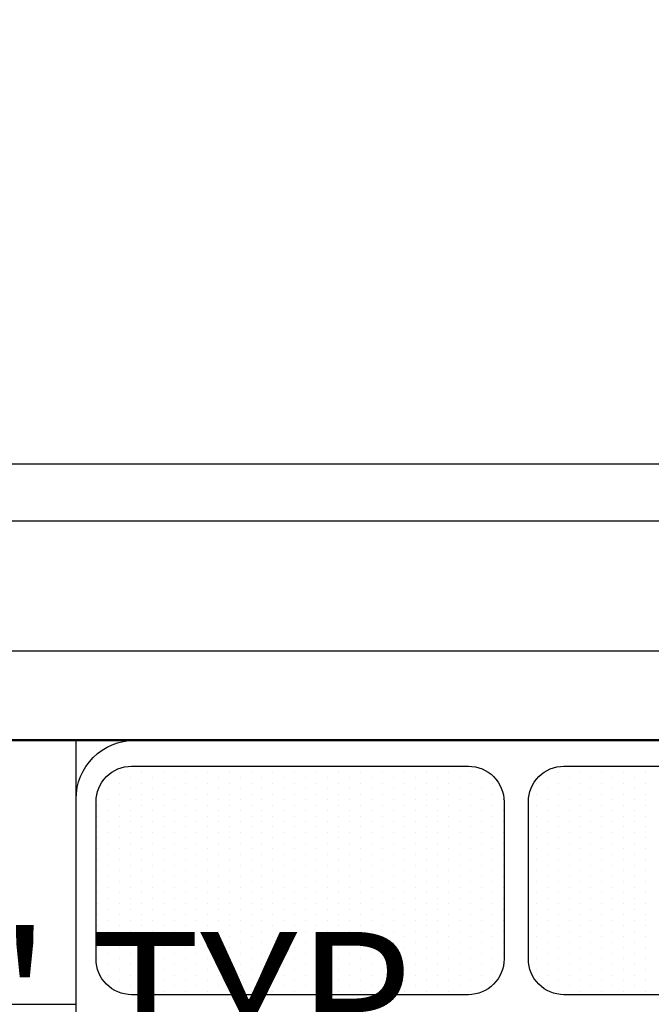
# Model space of a CAD drawing. Units: inches. Extents: x 3064 to 19385, y 846 to 15425.
# Tile 7 of 108: x 3426 to 3469, y 1373 to 1439. Entities that reach past the tile are written whole.
import ezdxf

# ---------------------------------------------------------------- set-up
doc = ezdxf.new("R2010")
doc.units = ezdxf.units.IN
for name, color, linetype, lineweight in [('A-ANNO-DIMS', 2, 'Continuous', 18), ('A-FLOR-FIXT', 9, 'Continuous', 18), ('A-WALL', 7, 'Continuous', 50), ('C-PROP', 6, 'Continuous', 25)]:
    doc.layers.add(name, color=color, linetype=linetype, lineweight=lineweight)
doc.layers.add('BLOCK', color=6, linetype='Continuous')
doc.styles.get("Standard").update_dxf_attribs({"font": 'arial.ttf'})
doc.dimstyles.new('ISO-25', dxfattribs={"dimtxt": 9, "dimasz": 2.5, "dimexe": 1.25, "dimexo": 0.625, "dimtad": 1, "dimdec": 1, "dimlunit": 3, "dimtxsty": 'Standard', "dimcen": 2.5, "dimadec": 0, "dimazin": 0, "dimtfac": 1, "dimtdec": 1, "dimtmove": 0, "dimatfit": 3, "dimfxl": 1, "dimarcsym": 0})

# ---------------------------------------------------------------- blocks, each defined once
blk = doc.blocks.new('*X7')
at = {"color": 0}
for p, q in [((266.25, 456.9375), (266.25, 456.9375)), ((266.4375, 457.03125), (266.4375, 457.03125)), ((266.625, 456.9375), (266.625, 456.9375)), ((266.8125, 457.03125), (266.8125, 457.03125)), ((267, 456.9375), (267, 456.9375)), ((267.1875, 457.03125), (267.1875, 457.03125)), ((267.375, 456.9375), (267.375, 456.9375)), ((267.5625, 457.03125), (267.5625, 457.03125)), ((267.75, 456.9375), (267.75, 456.9375)), ((267.9375, 457.03125), (267.9375, 457.03125)), ((268.125, 456.9375), (268.125, 456.9375)), ((268.3125, 457.03125), (268.3125, 457.03125)), ((268.5, 456.9375), (268.5, 456.9375)), ((268.6875, 457.03125), (268.6875, 457.03125)), ((268.875, 456.9375), (268.875, 456.9375)), ((269.0625, 457.03125), (269.0625, 457.03125)), ((269.25, 456.9375), (269.25, 456.9375)), ((269.4375, 457.03125), (269.4375, 457.03125)), ((269.625, 456.9375), (269.625, 456.9375)), ((269.8125, 457.03125), (269.8125, 457.03125)), ((270, 456.9375), (270, 456.9375)), ((270.1875, 457.03125), (270.1875, 457.03125)), ((270.375, 456.9375), (270.375, 456.9375)), ((270.5625, 457.03125), (270.5625, 457.03125)), ((270.75, 456.9375), (270.75, 456.9375)), ((270.9375, 457.03125), (270.9375, 457.03125)), ((271.125, 456.9375), (271.125, 456.9375)), ((271.3125, 457.03125), (271.3125, 457.03125)), ((271.5, 456.9375), (271.5, 456.9375)), ((271.6875, 457.03125), (271.6875, 457.03125)), ((271.875, 456.9375), (271.875, 456.9375)), ((272.0625, 457.03125), (272.0625, 457.03125)), ((272.25, 456.9375), (272.25, 456.9375)), ((273.75, 456.9375), (273.75, 456.9375)), ((273.9375, 457.03125), (273.9375, 457.03125)), ((274.125, 456.9375), (274.125, 456.9375)), ((274.3125, 457.03125), (274.3125, 457.03125)), ((274.5, 456.9375), (274.5, 456.9375)), ((274.6875, 457.03125), (274.6875, 457.03125)), ((274.875, 456.9375), (274.875, 456.9375)), ((275.0625, 457.03125), (275.0625, 457.03125)), ((275.25, 456.9375), (275.25, 456.9375)), ((266.0625, 456.84375), (266.0625, 456.84375)), ((266.25, 456.75), (266.25, 456.75)), ((266.4375, 456.84375), (266.4375, 456.84375)), ((266.625, 456.75), (266.625, 456.75)), ((266.8125, 456.84375), (266.8125, 456.84375)), ((267, 456.75), (267, 456.75)), ((267.1875, 456.84375), (267.1875, 456.84375)), ((267.375, 456.75), (267.375, 456.75)), ((267.5625, 456.84375), (267.5625, 456.84375)), ((267.75, 456.75), (267.75, 456.75)), ((267.9375, 456.84375), (267.9375, 456.84375)), ((268.125, 456.75), (268.125, 456.75)), ((268.3125, 456.84375), (268.3125, 456.84375)), ((268.5, 456.75), (268.5, 456.75)), ((268.6875, 456.84375), (268.6875, 456.84375)), ((268.875, 456.75), (268.875, 456.75)), ((269.0625, 456.84375), (269.0625, 456.84375)), ((269.25, 456.75), (269.25, 456.75)), ((269.4375, 456.84375), (269.4375, 456.84375)), ((269.625, 456.75), (269.625, 456.75)), ((269.8125, 456.84375), (269.8125, 456.84375)), ((270, 456.75), (270, 456.75)), ((270.1875, 456.84375), (270.1875, 456.84375)), ((270.375, 456.75), (270.375, 456.75)), ((270.5625, 456.84375), (270.5625, 456.84375)), ((270.75, 456.75), (270.75, 456.75)), ((270.9375, 456.84375), (270.9375, 456.84375)), ((271.125, 456.75), (271.125, 456.75)), ((271.3125, 456.84375), (271.3125, 456.84375)), ((271.5, 456.75), (271.5, 456.75)), ((271.6875, 456.84375), (271.6875, 456.84375)), ((271.875, 456.75), (271.875, 456.75)), ((272.0625, 456.84375), (272.0625, 456.84375)), ((272.25, 456.75), (272.25, 456.75)), ((272.4375, 456.84375), (272.4375, 456.84375)), ((272.625, 456.75), (272.625, 456.75)), ((273.375, 456.75), (273.375, 456.75)), ((273.5625, 456.84375), (273.5625, 456.84375)), ((273.75, 456.75), (273.75, 456.75)), ((273.9375, 456.84375), (273.9375, 456.84375)), ((274.125, 456.75), (274.125, 456.75)), ((274.3125, 456.84375), (274.3125, 456.84375)), ((274.5, 456.75), (274.5, 456.75)), ((274.6875, 456.84375), (274.6875, 456.84375)), ((274.875, 456.75), (274.875, 456.75)), ((275.0625, 456.84375), (275.0625, 456.84375)), ((275.25, 456.75), (275.25, 456.75)), ((265.875, 456.5625), (265.875, 456.5625)), ((266.0625, 456.65625), (266.0625, 456.65625)), ((266.25, 456.5625), (266.25, 456.5625)), ((266.4375, 456.65625), (266.4375, 456.65625)), ((266.625, 456.5625), (266.625, 456.5625)), ((266.8125, 456.65625), (266.8125, 456.65625)), ((267, 456.5625), (267, 456.5625)), ((267.1875, 456.65625), (267.1875, 456.65625)), ((267.375, 456.5625), (267.375, 456.5625)), ((267.5625, 456.65625), (267.5625, 456.65625)), ((267.75, 456.5625), (267.75, 456.5625)), ((267.9375, 456.65625), (267.9375, 456.65625)), ((268.125, 456.5625), (268.125, 456.5625)), ((268.3125, 456.65625), (268.3125, 456.65625)), ((268.5, 456.5625), (268.5, 456.5625)), ((268.6875, 456.65625), (268.6875, 456.65625)), ((268.875, 456.5625), (268.875, 456.5625)), ((269.0625, 456.65625), (269.0625, 456.65625)), ((269.25, 456.5625), (269.25, 456.5625)), ((269.4375, 456.65625), (269.4375, 456.65625)), ((269.625, 456.5625), (269.625, 456.5625)), ((269.8125, 456.65625), (269.8125, 456.65625)), ((270, 456.5625), (270, 456.5625)), ((270.1875, 456.65625), (270.1875, 456.65625)), ((270.375, 456.5625), (270.375, 456.5625)), ((270.5625, 456.65625), (270.5625, 456.65625)), ((270.75, 456.5625), (270.75, 456.5625)), ((270.9375, 456.65625), (270.9375, 456.65625)), ((271.125, 456.5625), (271.125, 456.5625)), ((271.3125, 456.65625), (271.3125, 456.65625)), ((271.5, 456.5625), (271.5, 456.5625)), ((271.6875, 456.65625), (271.6875, 456.65625)), ((271.875, 456.5625), (271.875, 456.5625)), ((272.0625, 456.65625), (272.0625, 456.65625)), ((272.25, 456.5625), (272.25, 456.5625)), ((272.4375, 456.65625), (272.4375, 456.65625)), ((272.625, 456.5625), (272.625, 456.5625)), ((273.375, 456.5625), (273.375, 456.5625)), ((273.5625, 456.65625), (273.5625, 456.65625)), ((273.75, 456.5625), (273.75, 456.5625)), ((273.9375, 456.65625), (273.9375, 456.65625)), ((274.125, 456.5625), (274.125, 456.5625)), ((274.3125, 456.65625), (274.3125, 456.65625)), ((274.5, 456.5625), (274.5, 456.5625)), ((274.6875, 456.65625), (274.6875, 456.65625)), ((274.875, 456.5625), (274.875, 456.5625)), ((275.0625, 456.65625), (275.0625, 456.65625)), ((275.25, 456.5625), (275.25, 456.5625)), ((265.875, 456.375), (265.875, 456.375)), ((266.0625, 456.46875), (266.0625, 456.46875)), ((266.25, 456.375), (266.25, 456.375)), ((266.4375, 456.46875), (266.4375, 456.46875)), ((266.625, 456.375), (266.625, 456.375)), ((266.8125, 456.46875), (266.8125, 456.46875)), ((267, 456.375), (267, 456.375)), ((267.1875, 456.46875), (267.1875, 456.46875)), ((267.375, 456.375), (267.375, 456.375)), ((267.5625, 456.46875), (267.5625, 456.46875)), ((267.75, 456.375), (267.75, 456.375)), ((267.9375, 456.46875), (267.9375, 456.46875)), ((268.125, 456.375), (268.125, 456.375)), ((268.3125, 456.46875), (268.3125, 456.46875)), ((268.5, 456.375), (268.5, 456.375)), ((268.6875, 456.46875), (268.6875, 456.46875)), ((268.875, 456.375), (268.875, 456.375)), ((269.0625, 456.46875), (269.0625, 456.46875)), ((269.25, 456.375), (269.25, 456.375)), ((269.4375, 456.46875), (269.4375, 456.46875)), ((269.625, 456.375), (269.625, 456.375)), ((269.8125, 456.46875), (269.8125, 456.46875)), ((270, 456.375), (270, 456.375)), ((270.1875, 456.46875), (270.1875, 456.46875)), ((270.375, 456.375), (270.375, 456.375)), ((270.5625, 456.46875), (270.5625, 456.46875)), ((270.75, 456.375), (270.75, 456.375)), ((270.9375, 456.46875), (270.9375, 456.46875)), ((271.125, 456.375), (271.125, 456.375)), ((271.3125, 456.46875), (271.3125, 456.46875)), ((271.5, 456.375), (271.5, 456.375)), ((271.6875, 456.46875), (271.6875, 456.46875)), ((271.875, 456.375), (271.875, 456.375)), ((272.0625, 456.46875), (272.0625, 456.46875)), ((272.25, 456.375), (272.25, 456.375)), ((272.4375, 456.46875), (272.4375, 456.46875)), ((272.625, 456.375), (272.625, 456.375)), ((272.8125, 456.46875), (272.8125, 456.46875)), ((273.375, 456.375), (273.375, 456.375)), ((273.5625, 456.46875), (273.5625, 456.46875)), ((273.75, 456.375), (273.75, 456.375)), ((273.9375, 456.46875), (273.9375, 456.46875)), ((274.125, 456.375), (274.125, 456.375)), ((274.3125, 456.46875), (274.3125, 456.46875)), ((274.5, 456.375), (274.5, 456.375)), ((274.6875, 456.46875), (274.6875, 456.46875)), ((274.875, 456.375), (274.875, 456.375)), ((275.0625, 456.46875), (275.0625, 456.46875)), ((275.25, 456.375), (275.25, 456.375)), ((266.0625, 456.28125), (266.0625, 456.28125)), ((266.4375, 456.28125), (266.4375, 456.28125)), ((266.8125, 456.28125), (266.8125, 456.28125)), ((267.1875, 456.28125), (267.1875, 456.28125)), ((267.5625, 456.28125), (267.5625, 456.28125)), ((267.9375, 456.28125), (267.9375, 456.28125)), ((268.3125, 456.28125), (268.3125, 456.28125)), ((268.6875, 456.28125), (268.6875, 456.28125)), ((269.0625, 456.28125), (269.0625, 456.28125)), ((269.4375, 456.28125), (269.4375, 456.28125)), ((269.8125, 456.28125), (269.8125, 456.28125)), ((270.1875, 456.28125), (270.1875, 456.28125)), ((270.5625, 456.28125), (270.5625, 456.28125)), ((270.9375, 456.28125), (270.9375, 456.28125)), ((271.3125, 456.28125), (271.3125, 456.28125)), ((271.6875, 456.28125), (271.6875, 456.28125)), ((272.0625, 456.28125), (272.0625, 456.28125)), ((272.4375, 456.28125), (272.4375, 456.28125)), ((272.8125, 456.28125), (272.8125, 456.28125)), ((273.5625, 456.28125), (273.5625, 456.28125)), ((273.9375, 456.28125), (273.9375, 456.28125)), ((274.3125, 456.28125), (274.3125, 456.28125)), ((274.6875, 456.28125), (274.6875, 456.28125)), ((275.0625, 456.28125), (275.0625, 456.28125)), ((265.875, 456.1875), (265.875, 456.1875)), ((266.0625, 456.09375), (266.0625, 456.09375)), ((266.25, 456.1875), (266.25, 456.1875)), ((266.4375, 456.09375), (266.4375, 456.09375)), ((266.625, 456.1875), (266.625, 456.1875)), ((266.8125, 456.09375), (266.8125, 456.09375)), ((267, 456.1875), (267, 456.1875)), ((267.1875, 456.09375), (267.1875, 456.09375)), ((267.375, 456.1875), (267.375, 456.1875)), ((267.5625, 456.09375), (267.5625, 456.09375)), ((267.75, 456.1875), (267.75, 456.1875)), ((267.9375, 456.09375), (267.9375, 456.09375)), ((268.125, 456.1875), (268.125, 456.1875)), ((268.3125, 456.09375), (268.3125, 456.09375)), ((268.5, 456.1875), (268.5, 456.1875)), ((268.6875, 456.09375), (268.6875, 456.09375)), ((268.875, 456.1875), (268.875, 456.1875)), ((269.0625, 456.09375), (269.0625, 456.09375)), ((269.25, 456.1875), (269.25, 456.1875)), ((269.4375, 456.09375), (269.4375, 456.09375)), ((269.625, 456.1875), (269.625, 456.1875)), ((269.8125, 456.09375), (269.8125, 456.09375)), ((270, 456.1875), (270, 456.1875)), ((270.1875, 456.09375), (270.1875, 456.09375)), ((270.375, 456.1875), (270.375, 456.1875)), ((270.5625, 456.09375), (270.5625, 456.09375)), ((270.75, 456.1875), (270.75, 456.1875)), ((270.9375, 456.09375), (270.9375, 456.09375)), ((271.125, 456.1875), (271.125, 456.1875)), ((271.3125, 456.09375), (271.3125, 456.09375)), ((271.5, 456.1875), (271.5, 456.1875)), ((271.6875, 456.09375), (271.6875, 456.09375)), ((271.875, 456.1875), (271.875, 456.1875)), ((272.0625, 456.09375), (272.0625, 456.09375)), ((272.25, 456.1875), (272.25, 456.1875)), ((272.4375, 456.09375), (272.4375, 456.09375)), ((272.625, 456.1875), (272.625, 456.1875)), ((272.8125, 456.09375), (272.8125, 456.09375)), ((273.375, 456.1875), (273.375, 456.1875)), ((273.5625, 456.09375), (273.5625, 456.09375)), ((273.75, 456.1875), (273.75, 456.1875)), ((273.9375, 456.09375), (273.9375, 456.09375)), ((274.125, 456.1875), (274.125, 456.1875)), ((274.3125, 456.09375), (274.3125, 456.09375)), ((274.5, 456.1875), (274.5, 456.1875)), ((274.6875, 456.09375), (274.6875, 456.09375)), ((274.875, 456.1875), (274.875, 456.1875)), ((275.0625, 456.09375), (275.0625, 456.09375)), ((275.25, 456.1875), (275.25, 456.1875)), ((265.875, 456), (265.875, 456)), ((266.0625, 455.90625), (266.0625, 455.90625)), ((266.25, 456), (266.25, 456)), ((266.4375, 455.90625), (266.4375, 455.90625)), ((266.625, 456), (266.625, 456)), ((266.8125, 455.90625), (266.8125, 455.90625)), ((267, 456), (267, 456)), ((267.1875, 455.90625), (267.1875, 455.90625)), ((267.375, 456), (267.375, 456)), ((267.5625, 455.90625), (267.5625, 455.90625)), ((267.75, 456), (267.75, 456)), ((267.9375, 455.90625), (267.9375, 455.90625)), ((268.125, 456), (268.125, 456)), ((268.3125, 455.90625), (268.3125, 455.90625)), ((268.5, 456), (268.5, 456)), ((268.6875, 455.90625), (268.6875, 455.90625)), ((268.875, 456), (268.875, 456)), ((269.0625, 455.90625), (269.0625, 455.90625)), ((269.25, 456), (269.25, 456)), ((269.4375, 455.90625), (269.4375, 455.90625)), ((269.625, 456), (269.625, 456)), ((269.8125, 455.90625), (269.8125, 455.90625)), ((270, 456), (270, 456)), ((270.1875, 455.90625), (270.1875, 455.90625)), ((270.375, 456), (270.375, 456)), ((270.5625, 455.90625), (270.5625, 455.90625)), ((270.75, 456), (270.75, 456)), ((270.9375, 455.90625), (270.9375, 455.90625)), ((271.125, 456), (271.125, 456)), ((271.3125, 455.90625), (271.3125, 455.90625)), ((271.5, 456), (271.5, 456)), ((271.6875, 455.90625), (271.6875, 455.90625)), ((271.875, 456), (271.875, 456)), ((272.0625, 455.90625), (272.0625, 455.90625)), ((272.25, 456), (272.25, 456)), ((272.4375, 455.90625), (272.4375, 455.90625)), ((272.625, 456), (272.625, 456)), ((272.8125, 455.90625), (272.8125, 455.90625)), ((273.375, 456), (273.375, 456)), ((273.5625, 455.90625), (273.5625, 455.90625)), ((273.75, 456), (273.75, 456)), ((273.9375, 455.90625), (273.9375, 455.90625)), ((274.125, 456), (274.125, 456)), ((274.3125, 455.90625), (274.3125, 455.90625)), ((274.5, 456), (274.5, 456)), ((274.6875, 455.90625), (274.6875, 455.90625)), ((274.875, 456), (274.875, 456)), ((275.0625, 455.90625), (275.0625, 455.90625)), ((275.25, 456), (275.25, 456)), ((265.875, 455.8125), (265.875, 455.8125)), ((266.0625, 455.71875), (266.0625, 455.71875)), ((266.25, 455.8125), (266.25, 455.8125)), ((266.4375, 455.71875), (266.4375, 455.71875)), ((266.625, 455.8125), (266.625, 455.8125)), ((266.8125, 455.71875), (266.8125, 455.71875)), ((267, 455.8125), (267, 455.8125)), ((267.1875, 455.71875), (267.1875, 455.71875)), ((267.375, 455.8125), (267.375, 455.8125)), ((267.5625, 455.71875), (267.5625, 455.71875)), ((267.75, 455.8125), (267.75, 455.8125)), ((267.9375, 455.71875), (267.9375, 455.71875)), ((268.125, 455.8125), (268.125, 455.8125)), ((268.3125, 455.71875), (268.3125, 455.71875)), ((268.5, 455.8125), (268.5, 455.8125)), ((268.6875, 455.71875), (268.6875, 455.71875)), ((268.875, 455.8125), (268.875, 455.8125)), ((269.0625, 455.71875), (269.0625, 455.71875)), ((269.25, 455.8125), (269.25, 455.8125)), ((269.4375, 455.71875), (269.4375, 455.71875)), ((269.625, 455.8125), (269.625, 455.8125)), ((269.8125, 455.71875), (269.8125, 455.71875)), ((270, 455.8125), (270, 455.8125)), ((270.1875, 455.71875), (270.1875, 455.71875)), ((270.375, 455.8125), (270.375, 455.8125)), ((270.5625, 455.71875), (270.5625, 455.71875)), ((270.75, 455.8125), (270.75, 455.8125)), ((270.9375, 455.71875), (270.9375, 455.71875)), ((271.125, 455.8125), (271.125, 455.8125)), ((271.3125, 455.71875), (271.3125, 455.71875)), ((271.5, 455.8125), (271.5, 455.8125)), ((271.6875, 455.71875), (271.6875, 455.71875)), ((271.875, 455.8125), (271.875, 455.8125)), ((272.0625, 455.71875), (272.0625, 455.71875)), ((272.25, 455.8125), (272.25, 455.8125)), ((272.4375, 455.71875), (272.4375, 455.71875)), ((272.625, 455.8125), (272.625, 455.8125)), ((272.8125, 455.71875), (272.8125, 455.71875)), ((273.375, 455.8125), (273.375, 455.8125)), ((273.5625, 455.71875), (273.5625, 455.71875)), ((273.75, 455.8125), (273.75, 455.8125)), ((273.9375, 455.71875), (273.9375, 455.71875)), ((274.125, 455.8125), (274.125, 455.8125)), ((274.3125, 455.71875), (274.3125, 455.71875)), ((274.5, 455.8125), (274.5, 455.8125)), ((274.6875, 455.71875), (274.6875, 455.71875)), ((274.875, 455.8125), (274.875, 455.8125)), ((275.0625, 455.71875), (275.0625, 455.71875)), ((275.25, 455.8125), (275.25, 455.8125)), ((265.875, 455.625), (265.875, 455.625)), ((266.0625, 455.53125), (266.0625, 455.53125)), ((266.25, 455.625), (266.25, 455.625)), ((266.4375, 455.53125), (266.4375, 455.53125)), ((266.625, 455.625), (266.625, 455.625)), ((266.8125, 455.53125), (266.8125, 455.53125)), ((267, 455.625), (267, 455.625)), ((267.1875, 455.53125), (267.1875, 455.53125)), ((267.375, 455.625), (267.375, 455.625)), ((267.5625, 455.53125), (267.5625, 455.53125)), ((267.75, 455.625), (267.75, 455.625)), ((267.9375, 455.53125), (267.9375, 455.53125)), ((268.125, 455.625), (268.125, 455.625)), ((268.3125, 455.53125), (268.3125, 455.53125)), ((268.5, 455.625), (268.5, 455.625)), ((268.6875, 455.53125), (268.6875, 455.53125)), ((268.875, 455.625), (268.875, 455.625)), ((269.0625, 455.53125), (269.0625, 455.53125)), ((269.25, 455.625), (269.25, 455.625)), ((269.4375, 455.53125), (269.4375, 455.53125)), ((269.625, 455.625), (269.625, 455.625)), ((269.8125, 455.53125), (269.8125, 455.53125)), ((270, 455.625), (270, 455.625)), ((270.1875, 455.53125), (270.1875, 455.53125)), ((270.375, 455.625), (270.375, 455.625)), ((270.5625, 455.53125), (270.5625, 455.53125)), ((270.75, 455.625), (270.75, 455.625)), ((270.9375, 455.53125), (270.9375, 455.53125)), ((271.125, 455.625), (271.125, 455.625)), ((271.3125, 455.53125), (271.3125, 455.53125)), ((271.5, 455.625), (271.5, 455.625)), ((271.6875, 455.53125), (271.6875, 455.53125)), ((271.875, 455.625), (271.875, 455.625)), ((272.0625, 455.53125), (272.0625, 455.53125)), ((272.25, 455.625), (272.25, 455.625)), ((272.4375, 455.53125), (272.4375, 455.53125)), ((272.625, 455.625), (272.625, 455.625)), ((272.8125, 455.53125), (272.8125, 455.53125)), ((273.375, 455.625), (273.375, 455.625)), ((273.5625, 455.53125), (273.5625, 455.53125)), ((273.75, 455.625), (273.75, 455.625)), ((273.9375, 455.53125), (273.9375, 455.53125)), ((274.125, 455.625), (274.125, 455.625)), ((274.3125, 455.53125), (274.3125, 455.53125)), ((274.5, 455.625), (274.5, 455.625)), ((274.6875, 455.53125), (274.6875, 455.53125)), ((274.875, 455.625), (274.875, 455.625)), ((275.0625, 455.53125), (275.0625, 455.53125)), ((275.25, 455.625), (275.25, 455.625)), ((265.875, 455.4375), (265.875, 455.4375)), ((266.25, 455.4375), (266.25, 455.4375)), ((266.625, 455.4375), (266.625, 455.4375)), ((267, 455.4375), (267, 455.4375)), ((267.375, 455.4375), (267.375, 455.4375)), ((267.75, 455.4375), (267.75, 455.4375)), ((268.125, 455.4375), (268.125, 455.4375)), ((268.5, 455.4375), (268.5, 455.4375)), ((268.875, 455.4375), (268.875, 455.4375)), ((269.25, 455.4375), (269.25, 455.4375)), ((269.625, 455.4375), (269.625, 455.4375)), ((270, 455.4375), (270, 455.4375)), ((270.375, 455.4375), (270.375, 455.4375)), ((270.75, 455.4375), (270.75, 455.4375)), ((271.125, 455.4375), (271.125, 455.4375)), ((271.5, 455.4375), (271.5, 455.4375)), ((271.875, 455.4375), (271.875, 455.4375)), ((272.25, 455.4375), (272.25, 455.4375)), ((272.625, 455.4375), (272.625, 455.4375)), ((273.375, 455.4375), (273.375, 455.4375)), ((273.75, 455.4375), (273.75, 455.4375)), ((274.125, 455.4375), (274.125, 455.4375)), ((274.5, 455.4375), (274.5, 455.4375)), ((274.875, 455.4375), (274.875, 455.4375)), ((275.25, 455.4375), (275.25, 455.4375)), ((265.875, 455.25), (265.875, 455.25)), ((266.0625, 455.34375), (266.0625, 455.34375)), ((266.25, 455.25), (266.25, 455.25)), ((266.4375, 455.34375), (266.4375, 455.34375)), ((266.625, 455.25), (266.625, 455.25)), ((266.8125, 455.34375), (266.8125, 455.34375)), ((267, 455.25), (267, 455.25)), ((267.1875, 455.34375), (267.1875, 455.34375)), ((267.375, 455.25), (267.375, 455.25)), ((267.5625, 455.34375), (267.5625, 455.34375)), ((267.75, 455.25), (267.75, 455.25)), ((267.9375, 455.34375), (267.9375, 455.34375)), ((268.125, 455.25), (268.125, 455.25)), ((268.3125, 455.34375), (268.3125, 455.34375)), ((268.5, 455.25), (268.5, 455.25)), ((268.6875, 455.34375), (268.6875, 455.34375)), ((268.875, 455.25), (268.875, 455.25)), ((269.0625, 455.34375), (269.0625, 455.34375)), ((269.25, 455.25), (269.25, 455.25)), ((269.4375, 455.34375), (269.4375, 455.34375)), ((269.625, 455.25), (269.625, 455.25)), ((269.8125, 455.34375), (269.8125, 455.34375)), ((270, 455.25), (270, 455.25)), ((270.1875, 455.34375), (270.1875, 455.34375)), ((270.375, 455.25), (270.375, 455.25)), ((270.5625, 455.34375), (270.5625, 455.34375)), ((270.75, 455.25), (270.75, 455.25)), ((270.9375, 455.34375), (270.9375, 455.34375)), ((271.125, 455.25), (271.125, 455.25)), ((271.3125, 455.34375), (271.3125, 455.34375)), ((271.5, 455.25), (271.5, 455.25)), ((271.6875, 455.34375), (271.6875, 455.34375)), ((271.875, 455.25), (271.875, 455.25)), ((272.0625, 455.34375), (272.0625, 455.34375)), ((272.25, 455.25), (272.25, 455.25)), ((272.4375, 455.34375), (272.4375, 455.34375)), ((272.625, 455.25), (272.625, 455.25)), ((272.8125, 455.34375), (272.8125, 455.34375)), ((273.375, 455.25), (273.375, 455.25)), ((273.5625, 455.34375), (273.5625, 455.34375)), ((273.75, 455.25), (273.75, 455.25)), ((273.9375, 455.34375), (273.9375, 455.34375)), ((274.125, 455.25), (274.125, 455.25)), ((274.3125, 455.34375), (274.3125, 455.34375)), ((274.5, 455.25), (274.5, 455.25)), ((274.6875, 455.34375), (274.6875, 455.34375)), ((274.875, 455.25), (274.875, 455.25)), ((275.0625, 455.34375), (275.0625, 455.34375)), ((275.25, 455.25), (275.25, 455.25)), ((265.875, 455.0625), (265.875, 455.0625)), ((266.0625, 455.15625), (266.0625, 455.15625)), ((266.25, 455.0625), (266.25, 455.0625)), ((266.4375, 455.15625), (266.4375, 455.15625)), ((266.625, 455.0625), (266.625, 455.0625)), ((266.8125, 455.15625), (266.8125, 455.15625)), ((267, 455.0625), (267, 455.0625)), ((267.1875, 455.15625), (267.1875, 455.15625)), ((267.375, 455.0625), (267.375, 455.0625)), ((267.5625, 455.15625), (267.5625, 455.15625)), ((267.75, 455.0625), (267.75, 455.0625)), ((267.9375, 455.15625), (267.9375, 455.15625)), ((268.125, 455.0625), (268.125, 455.0625)), ((268.3125, 455.15625), (268.3125, 455.15625)), ((268.5, 455.0625), (268.5, 455.0625)), ((268.6875, 455.15625), (268.6875, 455.15625)), ((268.875, 455.0625), (268.875, 455.0625)), ((269.0625, 455.15625), (269.0625, 455.15625)), ((269.25, 455.0625), (269.25, 455.0625)), ((269.4375, 455.15625), (269.4375, 455.15625)), ((269.625, 455.0625), (269.625, 455.0625)), ((269.8125, 455.15625), (269.8125, 455.15625)), ((270, 455.0625), (270, 455.0625)), ((270.1875, 455.15625), (270.1875, 455.15625)), ((270.375, 455.0625), (270.375, 455.0625)), ((270.5625, 455.15625), (270.5625, 455.15625)), ((270.75, 455.0625), (270.75, 455.0625)), ((270.9375, 455.15625), (270.9375, 455.15625)), ((271.125, 455.0625), (271.125, 455.0625)), ((271.3125, 455.15625), (271.3125, 455.15625)), ((271.5, 455.0625), (271.5, 455.0625)), ((271.6875, 455.15625), (271.6875, 455.15625)), ((271.875, 455.0625), (271.875, 455.0625)), ((272.0625, 455.15625), (272.0625, 455.15625)), ((272.25, 455.0625), (272.25, 455.0625)), ((272.4375, 455.15625), (272.4375, 455.15625)), ((272.625, 455.0625), (272.625, 455.0625)), ((272.8125, 455.15625), (272.8125, 455.15625)), ((273.375, 455.0625), (273.375, 455.0625)), ((273.5625, 455.15625), (273.5625, 455.15625)), ((273.75, 455.0625), (273.75, 455.0625)), ((273.9375, 455.15625), (273.9375, 455.15625)), ((274.125, 455.0625), (274.125, 455.0625)), ((274.3125, 455.15625), (274.3125, 455.15625)), ((274.5, 455.0625), (274.5, 455.0625)), ((274.6875, 455.15625), (274.6875, 455.15625)), ((274.875, 455.0625), (274.875, 455.0625)), ((275.0625, 455.15625), (275.0625, 455.15625)), ((275.25, 455.0625), (275.25, 455.0625)), ((265.875, 454.875), (265.875, 454.875)), ((266.0625, 454.96875), (266.0625, 454.96875)), ((266.25, 454.875), (266.25, 454.875)), ((266.4375, 454.96875), (266.4375, 454.96875)), ((266.625, 454.875), (266.625, 454.875)), ((266.8125, 454.96875), (266.8125, 454.96875)), ((267, 454.875), (267, 454.875)), ((267.1875, 454.96875), (267.1875, 454.96875)), ((267.375, 454.875), (267.375, 454.875)), ((267.5625, 454.96875), (267.5625, 454.96875)), ((267.75, 454.875), (267.75, 454.875)), ((267.9375, 454.96875), (267.9375, 454.96875)), ((268.125, 454.875), (268.125, 454.875)), ((268.3125, 454.96875), (268.3125, 454.96875)), ((268.5, 454.875), (268.5, 454.875)), ((268.6875, 454.96875), (268.6875, 454.96875)), ((268.875, 454.875), (268.875, 454.875)), ((269.0625, 454.96875), (269.0625, 454.96875)), ((269.25, 454.875), (269.25, 454.875)), ((269.4375, 454.96875), (269.4375, 454.96875)), ((269.625, 454.875), (269.625, 454.875)), ((269.8125, 454.96875), (269.8125, 454.96875)), ((270, 454.875), (270, 454.875)), ((270.1875, 454.96875), (270.1875, 454.96875)), ((270.375, 454.875), (270.375, 454.875)), ((270.5625, 454.96875), (270.5625, 454.96875)), ((270.75, 454.875), (270.75, 454.875)), ((270.9375, 454.96875), (270.9375, 454.96875)), ((271.125, 454.875), (271.125, 454.875)), ((271.3125, 454.96875), (271.3125, 454.96875)), ((271.5, 454.875), (271.5, 454.875)), ((271.6875, 454.96875), (271.6875, 454.96875)), ((271.875, 454.875), (271.875, 454.875)), ((272.0625, 454.96875), (272.0625, 454.96875)), ((272.25, 454.875), (272.25, 454.875)), ((272.4375, 454.96875), (272.4375, 454.96875)), ((272.625, 454.875), (272.625, 454.875)), ((272.8125, 454.96875), (272.8125, 454.96875)), ((273.375, 454.875), (273.375, 454.875)), ((273.5625, 454.96875), (273.5625, 454.96875)), ((273.75, 454.875), (273.75, 454.875)), ((273.9375, 454.96875), (273.9375, 454.96875)), ((274.125, 454.875), (274.125, 454.875)), ((274.3125, 454.96875), (274.3125, 454.96875)), ((274.5, 454.875), (274.5, 454.875)), ((274.6875, 454.96875), (274.6875, 454.96875)), ((274.875, 454.875), (274.875, 454.875)), ((275.0625, 454.96875), (275.0625, 454.96875)), ((275.25, 454.875), (275.25, 454.875)), ((265.875, 454.6875), (265.875, 454.6875)), ((266.0625, 454.78125), (266.0625, 454.78125)), ((266.25, 454.6875), (266.25, 454.6875)), ((266.4375, 454.78125), (266.4375, 454.78125)), ((266.625, 454.6875), (266.625, 454.6875)), ((266.8125, 454.78125), (266.8125, 454.78125)), ((267, 454.6875), (267, 454.6875)), ((267.1875, 454.78125), (267.1875, 454.78125)), ((267.375, 454.6875), (267.375, 454.6875)), ((267.5625, 454.78125), (267.5625, 454.78125)), ((267.75, 454.6875), (267.75, 454.6875)), ((267.9375, 454.78125), (267.9375, 454.78125)), ((268.125, 454.6875), (268.125, 454.6875)), ((268.3125, 454.78125), (268.3125, 454.78125)), ((268.5, 454.6875), (268.5, 454.6875)), ((268.6875, 454.78125), (268.6875, 454.78125)), ((268.875, 454.6875), (268.875, 454.6875)), ((269.0625, 454.78125), (269.0625, 454.78125)), ((269.25, 454.6875), (269.25, 454.6875)), ((269.4375, 454.78125), (269.4375, 454.78125)), ((269.625, 454.6875), (269.625, 454.6875)), ((269.8125, 454.78125), (269.8125, 454.78125)), ((270, 454.6875), (270, 454.6875)), ((270.1875, 454.78125), (270.1875, 454.78125)), ((270.375, 454.6875), (270.375, 454.6875)), ((270.5625, 454.78125), (270.5625, 454.78125)), ((270.75, 454.6875), (270.75, 454.6875)), ((270.9375, 454.78125), (270.9375, 454.78125)), ((271.125, 454.6875), (271.125, 454.6875)), ((271.3125, 454.78125), (271.3125, 454.78125)), ((271.5, 454.6875), (271.5, 454.6875)), ((271.6875, 454.78125), (271.6875, 454.78125)), ((271.875, 454.6875), (271.875, 454.6875)), ((272.0625, 454.78125), (272.0625, 454.78125)), ((272.25, 454.6875), (272.25, 454.6875)), ((272.4375, 454.78125), (272.4375, 454.78125)), ((272.625, 454.6875), (272.625, 454.6875)), ((272.8125, 454.78125), (272.8125, 454.78125)), ((273.375, 454.6875), (273.375, 454.6875)), ((273.5625, 454.78125), (273.5625, 454.78125)), ((273.75, 454.6875), (273.75, 454.6875)), ((273.9375, 454.78125), (273.9375, 454.78125)), ((274.125, 454.6875), (274.125, 454.6875)), ((274.3125, 454.78125), (274.3125, 454.78125)), ((274.5, 454.6875), (274.5, 454.6875)), ((274.6875, 454.78125), (274.6875, 454.78125)), ((274.875, 454.6875), (274.875, 454.6875)), ((275.0625, 454.78125), (275.0625, 454.78125)), ((275.25, 454.6875), (275.25, 454.6875)), ((266.0625, 454.59375), (266.0625, 454.59375)), ((266.4375, 454.59375), (266.4375, 454.59375)), ((266.8125, 454.59375), (266.8125, 454.59375)), ((267.1875, 454.59375), (267.1875, 454.59375)), ((267.5625, 454.59375), (267.5625, 454.59375)), ((267.9375, 454.59375), (267.9375, 454.59375)), ((268.3125, 454.59375), (268.3125, 454.59375)), ((268.6875, 454.59375), (268.6875, 454.59375)), ((269.0625, 454.59375), (269.0625, 454.59375)), ((269.4375, 454.59375), (269.4375, 454.59375)), ((269.8125, 454.59375), (269.8125, 454.59375)), ((270.1875, 454.59375), (270.1875, 454.59375)), ((270.5625, 454.59375), (270.5625, 454.59375)), ((270.9375, 454.59375), (270.9375, 454.59375)), ((271.3125, 454.59375), (271.3125, 454.59375)), ((271.6875, 454.59375), (271.6875, 454.59375)), ((272.0625, 454.59375), (272.0625, 454.59375)), ((272.4375, 454.59375), (272.4375, 454.59375)), ((272.8125, 454.59375), (272.8125, 454.59375)), ((273.5625, 454.59375), (273.5625, 454.59375)), ((273.9375, 454.59375), (273.9375, 454.59375)), ((274.3125, 454.59375), (274.3125, 454.59375)), ((274.6875, 454.59375), (274.6875, 454.59375)), ((275.0625, 454.59375), (275.0625, 454.59375)), ((265.875, 454.5), (265.875, 454.5)), ((266.0625, 454.40625), (266.0625, 454.40625)), ((266.25, 454.5), (266.25, 454.5)), ((266.4375, 454.40625), (266.4375, 454.40625)), ((266.625, 454.5), (266.625, 454.5)), ((266.8125, 454.40625), (266.8125, 454.40625)), ((267, 454.5), (267, 454.5)), ((267.1875, 454.40625), (267.1875, 454.40625)), ((267.375, 454.5), (267.375, 454.5)), ((267.5625, 454.40625), (267.5625, 454.40625)), ((267.75, 454.5), (267.75, 454.5)), ((267.9375, 454.40625), (267.9375, 454.40625)), ((268.125, 454.5), (268.125, 454.5)), ((268.3125, 454.40625), (268.3125, 454.40625)), ((268.5, 454.5), (268.5, 454.5)), ((268.6875, 454.40625), (268.6875, 454.40625)), ((268.875, 454.5), (268.875, 454.5)), ((269.0625, 454.40625), (269.0625, 454.40625)), ((269.25, 454.5), (269.25, 454.5)), ((269.4375, 454.40625), (269.4375, 454.40625)), ((269.625, 454.5), (269.625, 454.5)), ((269.8125, 454.40625), (269.8125, 454.40625)), ((270, 454.5), (270, 454.5)), ((270.1875, 454.40625), (270.1875, 454.40625)), ((270.375, 454.5), (270.375, 454.5)), ((270.5625, 454.40625), (270.5625, 454.40625)), ((270.75, 454.5), (270.75, 454.5)), ((270.9375, 454.40625), (270.9375, 454.40625)), ((271.125, 454.5), (271.125, 454.5)), ((271.3125, 454.40625), (271.3125, 454.40625)), ((271.5, 454.5), (271.5, 454.5)), ((271.6875, 454.40625), (271.6875, 454.40625)), ((271.875, 454.5), (271.875, 454.5)), ((272.0625, 454.40625), (272.0625, 454.40625)), ((272.25, 454.5), (272.25, 454.5)), ((272.4375, 454.40625), (272.4375, 454.40625)), ((272.625, 454.5), (272.625, 454.5)), ((272.8125, 454.40625), (272.8125, 454.40625)), ((273.375, 454.5), (273.375, 454.5)), ((273.5625, 454.40625), (273.5625, 454.40625)), ((273.75, 454.5), (273.75, 454.5)), ((273.9375, 454.40625), (273.9375, 454.40625)), ((274.125, 454.5), (274.125, 454.5)), ((274.3125, 454.40625), (274.3125, 454.40625)), ((274.5, 454.5), (274.5, 454.5)), ((274.6875, 454.40625), (274.6875, 454.40625)), ((274.875, 454.5), (274.875, 454.5)), ((275.0625, 454.40625), (275.0625, 454.40625)), ((275.25, 454.5), (275.25, 454.5)), ((265.875, 454.3125), (265.875, 454.3125)), ((266.0625, 454.21875), (266.0625, 454.21875)), ((266.25, 454.3125), (266.25, 454.3125)), ((266.4375, 454.21875), (266.4375, 454.21875)), ((266.625, 454.3125), (266.625, 454.3125)), ((266.8125, 454.21875), (266.8125, 454.21875)), ((267, 454.3125), (267, 454.3125)), ((267.1875, 454.21875), (267.1875, 454.21875)), ((267.375, 454.3125), (267.375, 454.3125)), ((267.5625, 454.21875), (267.5625, 454.21875)), ((267.75, 454.3125), (267.75, 454.3125)), ((267.9375, 454.21875), (267.9375, 454.21875)), ((268.125, 454.3125), (268.125, 454.3125)), ((268.3125, 454.21875), (268.3125, 454.21875)), ((268.5, 454.3125), (268.5, 454.3125)), ((268.6875, 454.21875), (268.6875, 454.21875)), ((268.875, 454.3125), (268.875, 454.3125)), ((269.0625, 454.21875), (269.0625, 454.21875)), ((269.25, 454.3125), (269.25, 454.3125)), ((269.4375, 454.21875), (269.4375, 454.21875)), ((269.625, 454.3125), (269.625, 454.3125)), ((269.8125, 454.21875), (269.8125, 454.21875)), ((270, 454.3125), (270, 454.3125)), ((270.1875, 454.21875), (270.1875, 454.21875)), ((270.375, 454.3125), (270.375, 454.3125)), ((270.5625, 454.21875), (270.5625, 454.21875)), ((270.75, 454.3125), (270.75, 454.3125)), ((270.9375, 454.21875), (270.9375, 454.21875)), ((271.125, 454.3125), (271.125, 454.3125)), ((271.3125, 454.21875), (271.3125, 454.21875)), ((271.5, 454.3125), (271.5, 454.3125)), ((271.6875, 454.21875), (271.6875, 454.21875)), ((271.875, 454.3125), (271.875, 454.3125)), ((272.0625, 454.21875), (272.0625, 454.21875)), ((272.25, 454.3125), (272.25, 454.3125)), ((272.4375, 454.21875), (272.4375, 454.21875)), ((272.625, 454.3125), (272.625, 454.3125)), ((272.8125, 454.21875), (272.8125, 454.21875)), ((273.375, 454.3125), (273.375, 454.3125)), ((273.5625, 454.21875), (273.5625, 454.21875)), ((273.75, 454.3125), (273.75, 454.3125)), ((273.9375, 454.21875), (273.9375, 454.21875)), ((274.125, 454.3125), (274.125, 454.3125)), ((274.3125, 454.21875), (274.3125, 454.21875)), ((274.5, 454.3125), (274.5, 454.3125)), ((274.6875, 454.21875), (274.6875, 454.21875)), ((274.875, 454.3125), (274.875, 454.3125)), ((275.0625, 454.21875), (275.0625, 454.21875)), ((275.25, 454.3125), (275.25, 454.3125)), ((265.875, 454.125), (265.875, 454.125)), ((266.0625, 454.03125), (266.0625, 454.03125)), ((266.25, 454.125), (266.25, 454.125)), ((266.4375, 454.03125), (266.4375, 454.03125)), ((266.625, 454.125), (266.625, 454.125)), ((266.8125, 454.03125), (266.8125, 454.03125)), ((267, 454.125), (267, 454.125)), ((267.1875, 454.03125), (267.1875, 454.03125)), ((267.375, 454.125), (267.375, 454.125)), ((267.5625, 454.03125), (267.5625, 454.03125)), ((267.75, 454.125), (267.75, 454.125)), ((267.9375, 454.03125), (267.9375, 454.03125)), ((268.125, 454.125), (268.125, 454.125)), ((268.3125, 454.03125), (268.3125, 454.03125)), ((268.5, 454.125), (268.5, 454.125)), ((268.6875, 454.03125), (268.6875, 454.03125)), ((268.875, 454.125), (268.875, 454.125)), ((269.0625, 454.03125), (269.0625, 454.03125)), ((269.25, 454.125), (269.25, 454.125)), ((269.4375, 454.03125), (269.4375, 454.03125)), ((269.625, 454.125), (269.625, 454.125)), ((269.8125, 454.03125), (269.8125, 454.03125)), ((270, 454.125), (270, 454.125)), ((270.1875, 454.03125), (270.1875, 454.03125)), ((270.375, 454.125), (270.375, 454.125)), ((270.5625, 454.03125), (270.5625, 454.03125)), ((270.75, 454.125), (270.75, 454.125)), ((270.9375, 454.03125), (270.9375, 454.03125)), ((271.125, 454.125), (271.125, 454.125)), ((271.3125, 454.03125), (271.3125, 454.03125)), ((271.5, 454.125), (271.5, 454.125)), ((271.6875, 454.03125), (271.6875, 454.03125)), ((271.875, 454.125), (271.875, 454.125)), ((272.0625, 454.03125), (272.0625, 454.03125)), ((272.25, 454.125), (272.25, 454.125)), ((272.4375, 454.03125), (272.4375, 454.03125)), ((272.625, 454.125), (272.625, 454.125)), ((272.8125, 454.03125), (272.8125, 454.03125)), ((273.375, 454.125), (273.375, 454.125)), ((273.5625, 454.03125), (273.5625, 454.03125)), ((273.75, 454.125), (273.75, 454.125)), ((273.9375, 454.03125), (273.9375, 454.03125)), ((274.125, 454.125), (274.125, 454.125)), ((274.3125, 454.03125), (274.3125, 454.03125)), ((274.5, 454.125), (274.5, 454.125)), ((274.6875, 454.03125), (274.6875, 454.03125)), ((274.875, 454.125), (274.875, 454.125)), ((275.0625, 454.03125), (275.0625, 454.03125)), ((275.25, 454.125), (275.25, 454.125)), ((265.875, 453.9375), (265.875, 453.9375)), ((266.25, 453.9375), (266.25, 453.9375)), ((266.625, 453.9375), (266.625, 453.9375)), ((267, 453.9375), (267, 453.9375)), ((267.375, 453.9375), (267.375, 453.9375)), ((267.75, 453.9375), (267.75, 453.9375)), ((268.125, 453.9375), (268.125, 453.9375)), ((268.5, 453.9375), (268.5, 453.9375)), ((268.875, 453.9375), (268.875, 453.9375)), ((269.25, 453.9375), (269.25, 453.9375)), ((269.625, 453.9375), (269.625, 453.9375)), ((270, 453.9375), (270, 453.9375)), ((270.375, 453.9375), (270.375, 453.9375)), ((270.75, 453.9375), (270.75, 453.9375)), ((271.125, 453.9375), (271.125, 453.9375)), ((271.5, 453.9375), (271.5, 453.9375)), ((271.875, 453.9375), (271.875, 453.9375)), ((272.25, 453.9375), (272.25, 453.9375)), ((272.625, 453.9375), (272.625, 453.9375)), ((273.375, 453.9375), (273.375, 453.9375)), ((273.75, 453.9375), (273.75, 453.9375)), ((274.125, 453.9375), (274.125, 453.9375)), ((274.5, 453.9375), (274.5, 453.9375)), ((274.875, 453.9375), (274.875, 453.9375)), ((275.25, 453.9375), (275.25, 453.9375)), ((265.875, 453.75), (265.875, 453.75)), ((266.0625, 453.84375), (266.0625, 453.84375)), ((266.25, 453.75), (266.25, 453.75)), ((266.4375, 453.84375), (266.4375, 453.84375)), ((266.625, 453.75), (266.625, 453.75)), ((266.8125, 453.84375), (266.8125, 453.84375)), ((267, 453.75), (267, 453.75)), ((267.1875, 453.84375), (267.1875, 453.84375)), ((267.375, 453.75), (267.375, 453.75)), ((267.5625, 453.84375), (267.5625, 453.84375)), ((267.75, 453.75), (267.75, 453.75)), ((267.9375, 453.84375), (267.9375, 453.84375)), ((268.125, 453.75), (268.125, 453.75)), ((268.3125, 453.84375), (268.3125, 453.84375)), ((268.5, 453.75), (268.5, 453.75)), ((268.6875, 453.84375), (268.6875, 453.84375)), ((268.875, 453.75), (268.875, 453.75)), ((269.0625, 453.84375), (269.0625, 453.84375)), ((269.25, 453.75), (269.25, 453.75)), ((269.4375, 453.84375), (269.4375, 453.84375)), ((269.625, 453.75), (269.625, 453.75)), ((269.8125, 453.84375), (269.8125, 453.84375)), ((270, 453.75), (270, 453.75)), ((270.1875, 453.84375), (270.1875, 453.84375)), ((270.375, 453.75), (270.375, 453.75)), ((270.5625, 453.84375), (270.5625, 453.84375)), ((270.75, 453.75), (270.75, 453.75)), ((270.9375, 453.84375), (270.9375, 453.84375)), ((271.125, 453.75), (271.125, 453.75)), ((271.3125, 453.84375), (271.3125, 453.84375)), ((271.5, 453.75), (271.5, 453.75)), ((271.6875, 453.84375), (271.6875, 453.84375)), ((271.875, 453.75), (271.875, 453.75)), ((272.0625, 453.84375), (272.0625, 453.84375)), ((272.25, 453.75), (272.25, 453.75)), ((272.4375, 453.84375), (272.4375, 453.84375)), ((272.625, 453.75), (272.625, 453.75)), ((272.8125, 453.84375), (272.8125, 453.84375)), ((273.375, 453.75), (273.375, 453.75)), ((273.5625, 453.84375), (273.5625, 453.84375)), ((273.75, 453.75), (273.75, 453.75)), ((273.9375, 453.84375), (273.9375, 453.84375)), ((274.125, 453.75), (274.125, 453.75)), ((274.3125, 453.84375), (274.3125, 453.84375)), ((274.5, 453.75), (274.5, 453.75)), ((274.6875, 453.84375), (274.6875, 453.84375)), ((274.875, 453.75), (274.875, 453.75)), ((275.0625, 453.84375), (275.0625, 453.84375)), ((275.25, 453.75), (275.25, 453.75)), ((266.0625, 453.65625), (266.0625, 453.65625)), ((266.25, 453.5625), (266.25, 453.5625)), ((266.4375, 453.65625), (266.4375, 453.65625)), ((266.625, 453.5625), (266.625, 453.5625)), ((266.8125, 453.65625), (266.8125, 453.65625)), ((267, 453.5625), (267, 453.5625)), ((267.1875, 453.65625), (267.1875, 453.65625)), ((267.375, 453.5625), (267.375, 453.5625)), ((267.5625, 453.65625), (267.5625, 453.65625)), ((267.75, 453.5625), (267.75, 453.5625)), ((267.9375, 453.65625), (267.9375, 453.65625)), ((268.125, 453.5625), (268.125, 453.5625)), ((268.3125, 453.65625), (268.3125, 453.65625)), ((268.5, 453.5625), (268.5, 453.5625)), ((268.6875, 453.65625), (268.6875, 453.65625)), ((268.875, 453.5625), (268.875, 453.5625)), ((269.0625, 453.65625), (269.0625, 453.65625)), ((269.25, 453.5625), (269.25, 453.5625)), ((269.4375, 453.65625), (269.4375, 453.65625)), ((269.625, 453.5625), (269.625, 453.5625)), ((269.8125, 453.65625), (269.8125, 453.65625)), ((270, 453.5625), (270, 453.5625)), ((270.1875, 453.65625), (270.1875, 453.65625)), ((270.375, 453.5625), (270.375, 453.5625)), ((270.5625, 453.65625), (270.5625, 453.65625)), ((270.75, 453.5625), (270.75, 453.5625)), ((270.9375, 453.65625), (270.9375, 453.65625)), ((271.125, 453.5625), (271.125, 453.5625)), ((271.3125, 453.65625), (271.3125, 453.65625)), ((271.5, 453.5625), (271.5, 453.5625)), ((271.6875, 453.65625), (271.6875, 453.65625)), ((271.875, 453.5625), (271.875, 453.5625)), ((272.0625, 453.65625), (272.0625, 453.65625)), ((272.25, 453.5625), (272.25, 453.5625)), ((272.4375, 453.65625), (272.4375, 453.65625)), ((272.625, 453.5625), (272.625, 453.5625)), ((272.8125, 453.65625), (272.8125, 453.65625)), ((273.375, 453.5625), (273.375, 453.5625)), ((273.5625, 453.65625), (273.5625, 453.65625)), ((273.75, 453.5625), (273.75, 453.5625)), ((273.9375, 453.65625), (273.9375, 453.65625)), ((274.125, 453.5625), (274.125, 453.5625)), ((274.3125, 453.65625), (274.3125, 453.65625)), ((274.5, 453.5625), (274.5, 453.5625)), ((274.6875, 453.65625), (274.6875, 453.65625)), ((274.875, 453.5625), (274.875, 453.5625)), ((275.0625, 453.65625), (275.0625, 453.65625)), ((275.25, 453.5625), (275.25, 453.5625)), ((266.0625, 453.46875), (266.0625, 453.46875)), ((266.25, 453.375), (266.25, 453.375)), ((266.4375, 453.46875), (266.4375, 453.46875)), ((266.625, 453.375), (266.625, 453.375)), ((266.8125, 453.46875), (266.8125, 453.46875)), ((267, 453.375), (267, 453.375)), ((267.1875, 453.46875), (267.1875, 453.46875)), ((267.375, 453.375), (267.375, 453.375)), ((267.5625, 453.46875), (267.5625, 453.46875)), ((267.75, 453.375), (267.75, 453.375)), ((267.9375, 453.46875), (267.9375, 453.46875)), ((268.125, 453.375), (268.125, 453.375)), ((268.3125, 453.46875), (268.3125, 453.46875)), ((268.5, 453.375), (268.5, 453.375)), ((268.6875, 453.46875), (268.6875, 453.46875)), ((268.875, 453.375), (268.875, 453.375)), ((269.0625, 453.46875), (269.0625, 453.46875)), ((269.25, 453.375), (269.25, 453.375)), ((269.4375, 453.46875), (269.4375, 453.46875)), ((269.625, 453.375), (269.625, 453.375)), ((269.8125, 453.46875), (269.8125, 453.46875)), ((270, 453.375), (270, 453.375)), ((270.1875, 453.46875), (270.1875, 453.46875)), ((270.375, 453.375), (270.375, 453.375)), ((270.5625, 453.46875), (270.5625, 453.46875)), ((270.75, 453.375), (270.75, 453.375)), ((270.9375, 453.46875), (270.9375, 453.46875)), ((271.125, 453.375), (271.125, 453.375)), ((271.3125, 453.46875), (271.3125, 453.46875)), ((271.5, 453.375), (271.5, 453.375)), ((271.6875, 453.46875), (271.6875, 453.46875)), ((271.875, 453.375), (271.875, 453.375)), ((272.0625, 453.46875), (272.0625, 453.46875)), ((272.25, 453.375), (272.25, 453.375)), ((272.4375, 453.46875), (272.4375, 453.46875)), ((272.625, 453.375), (272.625, 453.375)), ((273.375, 453.375), (273.375, 453.375)), ((273.5625, 453.46875), (273.5625, 453.46875)), ((273.75, 453.375), (273.75, 453.375)), ((273.9375, 453.46875), (273.9375, 453.46875)), ((274.125, 453.375), (274.125, 453.375)), ((274.3125, 453.46875), (274.3125, 453.46875)), ((274.5, 453.375), (274.5, 453.375)), ((274.6875, 453.46875), (274.6875, 453.46875)), ((274.875, 453.375), (274.875, 453.375)), ((275.0625, 453.46875), (275.0625, 453.46875)), ((275.25, 453.375), (275.25, 453.375)), ((266.0625, 453.28125), (266.0625, 453.28125)), ((266.25, 453.1875), (266.25, 453.1875)), ((266.4375, 453.28125), (266.4375, 453.28125)), ((266.625, 453.1875), (266.625, 453.1875)), ((266.8125, 453.28125), (266.8125, 453.28125)), ((267, 453.1875), (267, 453.1875)), ((267.1875, 453.28125), (267.1875, 453.28125)), ((267.375, 453.1875), (267.375, 453.1875)), ((267.5625, 453.28125), (267.5625, 453.28125)), ((267.75, 453.1875), (267.75, 453.1875)), ((267.9375, 453.28125), (267.9375, 453.28125)), ((268.125, 453.1875), (268.125, 453.1875)), ((268.3125, 453.28125), (268.3125, 453.28125)), ((268.5, 453.1875), (268.5, 453.1875)), ((268.6875, 453.28125), (268.6875, 453.28125)), ((268.875, 453.1875), (268.875, 453.1875)), ((269.0625, 453.28125), (269.0625, 453.28125)), ((269.25, 453.1875), (269.25, 453.1875)), ((269.4375, 453.28125), (269.4375, 453.28125)), ((269.625, 453.1875), (269.625, 453.1875)), ((269.8125, 453.28125), (269.8125, 453.28125)), ((270, 453.1875), (270, 453.1875)), ((270.1875, 453.28125), (270.1875, 453.28125)), ((270.375, 453.1875), (270.375, 453.1875)), ((270.5625, 453.28125), (270.5625, 453.28125)), ((270.75, 453.1875), (270.75, 453.1875)), ((270.9375, 453.28125), (270.9375, 453.28125)), ((271.125, 453.1875), (271.125, 453.1875)), ((271.3125, 453.28125), (271.3125, 453.28125)), ((271.5, 453.1875), (271.5, 453.1875)), ((271.6875, 453.28125), (271.6875, 453.28125)), ((271.875, 453.1875), (271.875, 453.1875)), ((272.0625, 453.28125), (272.0625, 453.28125)), ((272.25, 453.1875), (272.25, 453.1875)), ((272.4375, 453.28125), (272.4375, 453.28125)), ((273.5625, 453.28125), (273.5625, 453.28125)), ((273.75, 453.1875), (273.75, 453.1875)), ((273.9375, 453.28125), (273.9375, 453.28125)), ((274.125, 453.1875), (274.125, 453.1875)), ((274.3125, 453.28125), (274.3125, 453.28125)), ((274.5, 453.1875), (274.5, 453.1875)), ((274.6875, 453.28125), (274.6875, 453.28125)), ((274.875, 453.1875), (274.875, 453.1875)), ((275.0625, 453.28125), (275.0625, 453.28125)), ((275.25, 453.1875), (275.25, 453.1875))]:
    blk.add_line(p, q, dxfattribs=at)
blk = doc.blocks.new('A$C52E67D0D')
at = {"layer": 'BLOCK'}
blk.add_lwpolyline([(501, 1348.6), (501, 1799.6), (0, 1799.6), (0, 1348.6)], close=True, dxfattribs=at)
for points in [[(1901, 0), (601, 0, -0.414214), (501, 100), (501, 1700, -0.414214), (601, 1800), (1901, 1800, -0.414214), (2001, 1700), (2001, 100, -0.414214)], [(1171.8, 1365.1), (595.8, 1365.1, -0.414214), (535, 1425.9), (535, 1694.8, -0.414214), (595.8, 1755.7), (1171.8, 1755.7, -0.414214), (1232.6, 1694.8), (1232.6, 1425.9, -0.414214)], [(1911, 1365.1), (1335, 1365.1, -0.414214), (1274.2, 1425.9), (1274.2, 1694.8, -0.414214), (1335, 1755.7), (1911, 1755.7, -0.414214), (1971.8, 1694.8), (1971.8, 1425.9, -0.414214)]]:
    blk.add_lwpolyline(points, format="xyb", close=True, dxfattribs=at)
blk.add_arc((1888.6, -1664.5), 3015.3, 87.8642, 117.4001, dxfattribs=at)
at = {"layer": 'BLOCK', "xscale": 100, "yscale": 100, "zscale": 100}
blk.add_blockref('*X7', (-26050, -43948.2), dxfattribs=at)
blk = doc.blocks.new('*D38')
at = {"layer": 'A-ANNO-DIMS', "color": 0, "lineweight": -2, "transparency": 16777216}
for p, q in [((3220.848, 1396.965), (3220.848, 1410.198)), ((3562.848, 1396.965), (3562.848, 1410.198)), ((3223.348, 1408.948), (3560.348, 1408.948))]:
    blk.add_line(p, q, dxfattribs=at)
at = {"layer": 'A-ANNO-DIMS', "color": 0, "transparency": 16777216}
for points in [[(3223.348, 1409.365), (3223.348, 1408.531), (3220.848, 1408.948)], [(3560.348, 1409.365), (3560.348, 1408.531), (3562.848, 1408.948)]]:
    blk.add_solid(points, dxfattribs=at)
at = {"layer": 'Defpoints', "color": 0, "transparency": 16777216}
for p in [(3562.848, 1408.948), (3220.848, 1396.34), (3562.848, 1396.34)]:
    blk.add_point(p, dxfattribs=at)
at = {"layer": 'A-ANNO-DIMS', "color": 0, "transparency": 16777216, "insert": (3391.848, 1414.168), "char_height": 9, "attachment_point": 5}
blk.add_mtext('28\'-6"', dxfattribs=at)
blk = doc.blocks.new('*D401')
at = {"layer": 'A-ANNO-DIMS', "color": 0, "lineweight": -2, "transparency": 16777216}
for p, q in [((3410.096, 1390.965), (3410.096, 1406.366)), ((3508.6, 1390.965), (3508.6, 1406.366)), ((3412.596, 1405.116), (3506.1, 1405.116)), ((3508.6, 1405.116), (3617.127, 1405.116))]:
    blk.add_line(p, q, dxfattribs=at)
at = {"layer": 'A-ANNO-DIMS', "color": 0, "transparency": 16777216}
for points in [[(3412.596, 1405.532), (3412.596, 1404.699), (3410.096, 1405.116)], [(3506.1, 1405.532), (3506.1, 1404.699), (3508.6, 1405.116)]]:
    blk.add_solid(points, dxfattribs=at)
at = {"layer": 'Defpoints', "color": 0, "transparency": 16777216}
for p in [(3508.6, 1405.116), (3410.096, 1390.34), (3508.6, 1390.34)]:
    blk.add_point(p, dxfattribs=at)
at = {"layer": 'A-ANNO-DIMS', "color": 0, "transparency": 16777216, "insert": (3564.114, 1410.394), "char_height": 9, "attachment_point": 5}
blk.add_mtext('BED 8\'-2 1/2" TYP.', dxfattribs=at)
blk = doc.blocks.new('*D427')
at = {"layer": 'A-ANNO-DIMS', "color": 0, "lineweight": -2, "transparency": 16777216}
for p, q in [((3296.059, 1369.474), (3296.059, 1365.249)), ((3320.059, 1369.474), (3320.059, 1365.249)), ((3298.559, 1366.499), (3317.559, 1366.499)), ((3320.059, 1366.499), (3460.682, 1366.499))]:
    blk.add_line(p, q, dxfattribs=at)
at = {"layer": 'A-ANNO-DIMS', "color": 0, "transparency": 16777216}
for points in [[(3298.559, 1366.915), (3298.559, 1366.082), (3296.059, 1366.499)], [(3317.559, 1366.915), (3317.559, 1366.082), (3320.059, 1366.499)]]:
    blk.add_solid(points, dxfattribs=at)
at = {"layer": 'Defpoints', "color": 0, "transparency": 16777216}
for p in [(3296.059, 1370.099), (3320.059, 1370.099), (3320.059, 1366.499)]:
    blk.add_point(p, dxfattribs=at)
at = {"layer": 'A-ANNO-DIMS', "color": 0, "transparency": 16777216, "insert": (3391.621, 1371.78), "char_height": 9, "attachment_point": 5}
blk.add_mtext('MICROWAVE 2\'-0" TYP.', dxfattribs=at)

msp = doc.modelspace()

# ---------------------------------------------------------------- linework, layer by layer
at = {"layer": 'A-WALL'}
msp.add_line((3556.848, 1390.34), (3361.848, 1390.34), dxfattribs=at)
at = {"layer": 'C-PROP'}
msp.add_line((3562.848, 1396.34), (3220.848, 1396.34), dxfattribs=at)

# ---------------------------------------------------------------- block references
at = {"layer": 'A-FLOR-FIXT', "xscale": 0.039370099999992, "yscale": 0.039370099999992, "zscale": 0.039370099999992}
msp.add_blockref('A$C52E67D0D', (3410.096, 1319.474), dxfattribs=at)

# ---------------------------------------------------------------- dimensions: what is measured, and where the dimension line sits
at = {"layer": 'A-ANNO-DIMS'}
for base, p1, p2, text, picture, middle in [((3508.6, 1405.116), (3410.096, 1390.34), (3508.6, 1390.34), 'BED <> TYP.', '*D401', (3564.114, 1410.394)), ((3320.059, 1366.499), (3296.059, 1370.099), (3320.059, 1370.099), 'MICROWAVE <> TYP.', '*D427', (3391.621, 1371.78))]:
    dim = msp.add_linear_dim(base=base, p1=p1, p2=p2, text=text, dimstyle='ISO-25', override={"dimdec": 1, "dimrnd": 0, "dimzin": 1, "dimlunit": 4, "dimfrac": 2}, dxfattribs=at)
    dim.commit()
    dim.dimension.update_dxf_attribs({"geometry": picture, "text_midpoint": middle})
dim = msp.add_linear_dim(base=(3562.848, 1408.948), p1=(3220.848, 1396.34), p2=(3562.848, 1396.34), dimstyle='ISO-25', override={"dimclrd": 0, "dimclre": 0, "dimclrt": 0}, dxfattribs=at)
dim.commit()
dim.dimension.update_dxf_attribs({"geometry": '*D38', "text_midpoint": (3391.848, 1414.168)})

doc.saveas('drawing.dxf')
